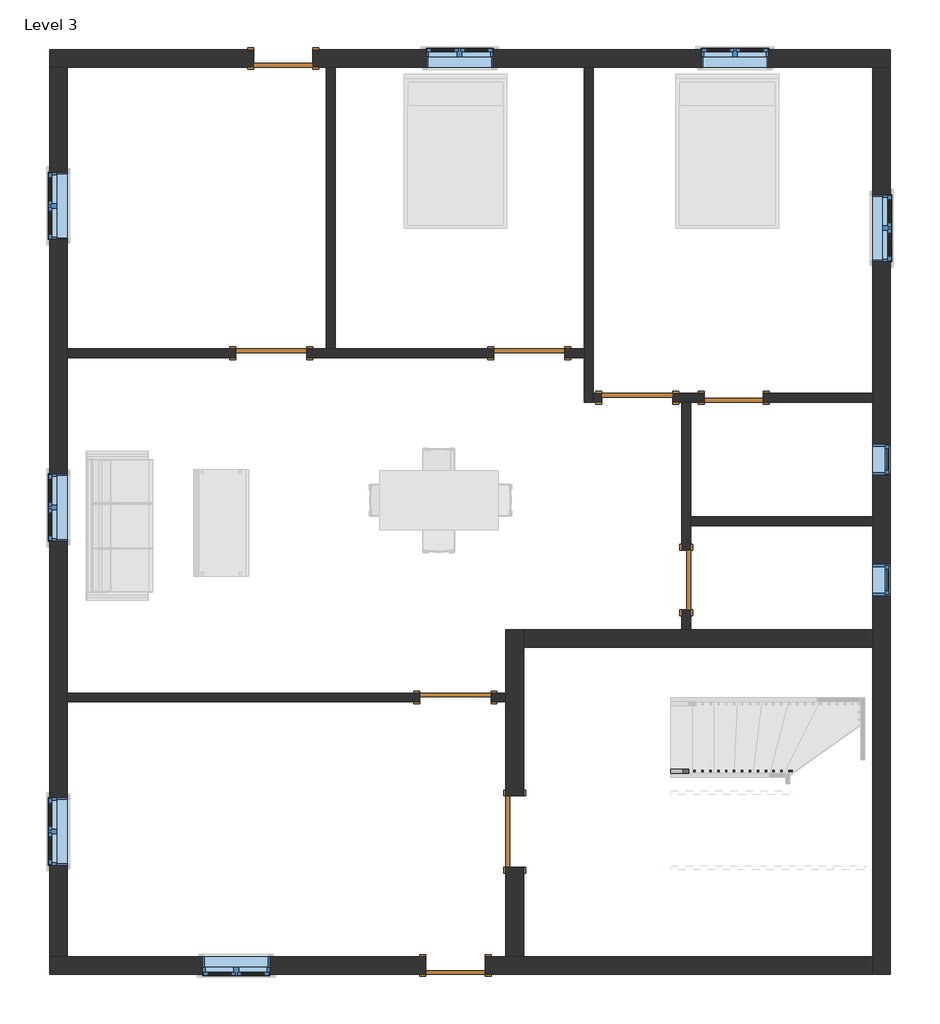
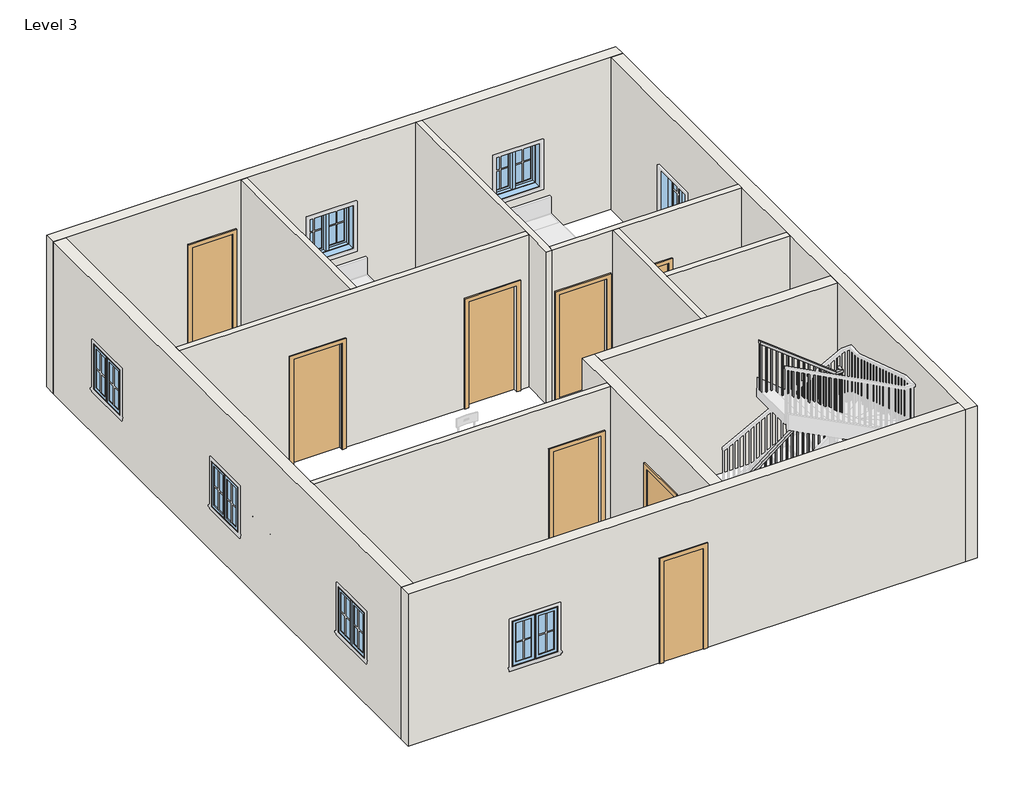
# One storey, part 1 of 2: 13 walls, 9 doors, 9 windows, 1 railing.
"""IFC4 building model written with IfcOpenShell, lengths in millimetres."""

from ifc_helpers import new_model, si_unit, frame, origin, place, context, project, spatial, polyline, outline, extrude, faceted_brep, transform, mapped, element, save
from components import door_85036156, door_d8f5dbb5, door_a1484949, door_e5f9f3c4, door_305aa2a5, door_0ca8825f, window_aa618e30, window_339605e1

model = new_model("IFC4")

# Units and contexts
model_context = context("Model", 3, world=origin())
ifc_project = project(units=[si_unit("LENGTHUNIT", "METRE", prefix="MILLI")], contexts=[model_context])

# Site, building, storey
site = spatial("IfcSite", under=ifc_project)
building = spatial("IfcBuilding", under=site)
storey = spatial("IfcBuildingStorey", under=building, Name="Level 3", Elevation=3200.4)

# Doors
placement = place(None, origin())
door_shape = door_85036156(model_context)
element("IfcDoor", 1, ObjectType="Single-Flush : 30\" x 80\"", at=placement, inside=storey, context=model_context, shape_type="MappedRepresentation", body=[
    mapped(door_shape, transform((-3639.3817864, 7024.9034997, 3200.4), x_axis=(1.0, 0.0, 0.0), y_axis=(0.0, 1.0, 0.0), z_axis=(0.0, 0.0, 1.0))),
])
door_2_shape = door_d8f5dbb5(model_context)
element("IfcDoor", 2, ObjectType="Single-Flush : 30\" x 80\"", at=placement, inside=storey, context=model_context, shape_type="MappedRepresentation", body=[
    mapped(door_2_shape, transform((2149.2782136, 2662.4534997, 3200.4), x_axis=(-1.0, 0.0, 0.0), y_axis=(0.0, -1.0, 0.0), z_axis=(0.0, 0.0, 1.0))),
])
element("IfcDoor", 3, ObjectType="Single-Flush : 30\" x 80\"", at=placement, inside=storey, context=model_context, shape_type="MappedRepresentation", body=[
    mapped(door_2_shape, transform((1539.6782136, 322.4784997, 3200.4), x_axis=(0.0, -1.0, 0.0), y_axis=(1.0, 0.0, 0.0), z_axis=(0.0, 0.0, 1.0))),
])
door_3_shape = door_a1484949(model_context)
element("IfcDoor", 4, ObjectType="Single-Flush : 30\" x 80\"", at=placement, inside=storey, context=model_context, shape_type="MappedRepresentation", body=[
    mapped(door_3_shape, transform((-1425.7717864, -4633.6965003, 3200.4), x_axis=(-1.0, 0.0, 0.0), y_axis=(0.0, -1.0, 0.0), z_axis=(0.0, 0.0, 1.0))),
])
door_4_shape = door_e5f9f3c4(model_context)
element("IfcDoor", 5, ObjectType="Single-Flush : 36\" x 84\"", at=placement, inside=storey, context=model_context, shape_type="MappedRepresentation", body=[
    mapped(door_4_shape, transform((-477.0817864, 3233.9534997, 3200.4), x_axis=(1.0, 0.0, 0.0), y_axis=(0.0, 1.0, 0.0), z_axis=(0.0, 0.0, 1.0))),
])
element("IfcDoor", 6, ObjectType="Single-Flush : 36\" x 84\"", at=placement, inside=storey, context=model_context, shape_type="MappedRepresentation", body=[
    mapped(door_4_shape, transform((-3791.7817864, 3233.9534997, 3200.4), x_axis=(1.0, 0.0, 0.0), y_axis=(0.0, 1.0, 0.0), z_axis=(0.0, 0.0, 1.0))),
])
element("IfcDoor", 7, ObjectType="Single-Flush : 36\" x 84\"", at=placement, inside=storey, context=model_context, shape_type="MappedRepresentation", body=[
    mapped(door_4_shape, transform((-1425.7717864, -1188.1865003, 3200.4), x_axis=(1.0, 0.0, 0.0), y_axis=(0.0, 1.0, 0.0), z_axis=(0.0, 0.0, 1.0))),
])
door_5_shape = door_305aa2a5(model_context)
element("IfcDoor", 8, ObjectType="Single-Flush : 36\" x 84\"", at=placement, inside=storey, context=model_context, shape_type="MappedRepresentation", body=[
    mapped(door_5_shape, transform((912.2982136, 2662.4534997, 3200.4), x_axis=(-1.0, 0.0, 0.0), y_axis=(0.0, -1.0, 0.0), z_axis=(0.0, 0.0, 1.0))),
])
door_6_shape = door_0ca8825f(model_context)
element("IfcDoor", 9, ObjectType="Single-Flush : 36\" x 84\"", at=placement, inside=storey, context=model_context, shape_type="MappedRepresentation", body=[
    mapped(door_6_shape, transform((-663.7717864, -2910.9415003, 3200.4), x_axis=(0.0, 1.0, 0.0), y_axis=(-1.0, 0.0, 0.0), z_axis=(0.0, 0.0, 1.0))),
])

# Railing
element("IfcRailing", 10, ObjectType="Handrail - Rectangular", at=placement, inside=storey, context=model_context, shape_type="SolidModel", body=[
    faceted_brep([(1342.8282136, -2108.9365003, 4284.1333333), (1342.8282136, -2108.9365003, 4219.8000346), (1342.8282136, -2159.7365003, 4219.8000346), (1342.8282136, -2159.7365003, 4284.1333333), (2794.3599055, -2108.9365003, 5412.0191036), (2845.1599055, -2108.9365003, 5387.1590024), (2845.1599055, -2159.7365003, 5387.1590024), (2794.3599055, -2159.7365003, 5412.0191036), (2794.3599055, -2108.9365003, 5615.0281882), (2845.1599055, -2108.9365003, 5564.2281882), (2845.1599055, -2159.7365003, 5564.2281882), (2794.3599055, -2159.7365003, 5615.0281882), (2921.3599055, -2108.9365003, 5615.0281882), (2921.3599055, -2108.9365003, 5564.2281882), (2870.5599055, -2159.7365003, 5564.2281882), (2870.5599055, -2159.7365003, 5615.0281882), (2921.3599055, -2235.9365003, 5615.0281882), (2921.3599055, -2265.0578342, 5564.2281882), (2870.5599055, -2265.0578342, 5564.2281882), (2870.5599055, -2235.9365003, 5615.0281882), (2921.3599055, -2362.9365003, 5831.9051451), (2921.3599055, -2413.7365003, 5818.1256424), (2870.5599055, -2413.7365003, 5818.1256424), (2870.5599055, -2362.9365003, 5831.9051451), (2921.3599055, -2362.9365003, 6034.9142297), (2921.3599055, -2413.7365003, 5984.1142297), (2870.5599055, -2413.7365003, 5984.1142297), (2870.5599055, -2362.9365003, 6034.9142297), (2921.3599055, -2489.9365003, 6034.9142297), (2921.3599055, -2489.9365003, 5984.1142297), (2870.5599055, -2439.1365003, 5984.1142297), (2870.5599055, -2439.1365003, 6034.9142297), (2794.3599055, -2489.9365003, 6034.9142297), (2776.9432376, -2489.9365003, 5984.1142297), (2776.9432376, -2439.1365003, 5984.1142297), (2794.3599055, -2439.1365003, 6034.9142297), (1342.8282136, -2489.9365003, 7162.8), (1342.8282136, -2439.1365003, 7162.8), (1342.8282136, -2439.1365003, 7098.4667013), (1342.8282136, -2489.9365003, 7098.4667013)], [[[0, 1, 2, 3]], [[1, 0, 4, 5]], [[2, 1, 5, 6]], [[3, 2, 6, 7]], [[0, 3, 7, 4]], [[5, 4, 8, 9]], [[6, 5, 9, 10]], [[7, 6, 10, 11]], [[4, 7, 11, 8]], [[9, 8, 12, 13]], [[10, 9, 13, 14]], [[11, 10, 14, 15]], [[8, 11, 15, 12]], [[13, 12, 16, 17]], [[14, 13, 17, 18]], [[15, 14, 18, 19]], [[12, 15, 19, 16]], [[17, 16, 20, 21]], [[18, 17, 21, 22]], [[19, 18, 22, 23]], [[16, 19, 23, 20]], [[21, 20, 24, 25]], [[22, 21, 25, 26]], [[23, 22, 26, 27]], [[20, 23, 27, 24]], [[25, 24, 28, 29]], [[26, 25, 29, 30]], [[27, 26, 30, 31]], [[24, 27, 31, 28]], [[29, 28, 32, 33]], [[30, 29, 33, 34]], [[31, 30, 34, 35]], [[28, 31, 35, 32]], [[36, 37, 38, 39]], [[33, 32, 36, 39]], [[34, 33, 39, 38]], [[35, 34, 38, 37]], [[32, 35, 37, 36]]]),
    extrude(outline(polyline([(7068.4292361, 1381.4849055), (7083.2316852, 1362.4349055), (6079.0666667, 1362.4349055), (6079.0666667, 1381.4849055), (7068.4292361, 1381.4849055)])), frame((0.0, -2474.0615003, 0.0), z_axis=(0.0, 1.0, 0.0), x_axis=(0.0, 0.0, 1.0)), (0.0, 0.0, 1.0), 19.05),
    extrude(outline(polyline([(6989.4828411, 1483.0849055), (7004.2852902, 1464.0349055), (6079.0666667, 1464.0349055), (6079.0666667, 1483.0849055), (6989.4828411, 1483.0849055)])), frame((0.0, -2474.0615003, 0.0), z_axis=(0.0, 1.0, 0.0), x_axis=(0.0, 0.0, 1.0)), (0.0, 0.0, 1.0), 19.05),
    extrude(outline(polyline([(6910.5364462, 1584.6849055), (6925.3388952, 1565.6349055), (6079.0666667, 1565.6349055), (6079.0666667, 1584.6849055), (6910.5364462, 1584.6849055)])), frame((0.0, -2474.0615003, 0.0), z_axis=(0.0, 1.0, 0.0), x_axis=(0.0, 0.0, 1.0)), (0.0, 0.0, 1.0), 19.05),
    extrude(outline(polyline([(6831.5900512, 1686.2849055), (6846.3925003, 1667.2349055), (5909.7333333, 1667.2349055), (5909.7333333, 1686.2849055), (6831.5900512, 1686.2849055)])), frame((0.0, -2474.0615003, 0.0), z_axis=(0.0, 1.0, 0.0), x_axis=(0.0, 0.0, 1.0)), (0.0, 0.0, 1.0), 19.05),
    extrude(outline(polyline([(6752.6436562, 1787.8849055), (6767.4461053, 1768.8349055), (5909.7333333, 1768.8349055), (5909.7333333, 1787.8849055), (6752.6436562, 1787.8849055)])), frame((0.0, -2474.0615003, 0.0), z_axis=(0.0, 1.0, 0.0), x_axis=(0.0, 0.0, 1.0)), (0.0, 0.0, 1.0), 19.05),
    extrude(outline(polyline([(6673.6972613, 1889.4849055), (6688.4997103, 1870.4349055), (5909.7333333, 1870.4349055), (5909.7333333, 1889.4849055), (6673.6972613, 1889.4849055)])), frame((0.0, -2474.0615003, 0.0), z_axis=(0.0, 1.0, 0.0), x_axis=(0.0, 0.0, 1.0)), (0.0, 0.0, 1.0), 19.05),
    extrude(outline(polyline([(6594.7508663, 1991.0849055), (6609.5533154, 1972.0349055), (5740.4, 1972.0349055), (5740.4, 1991.0849055), (6594.7508663, 1991.0849055)])), frame((0.0, -2474.0615003, 0.0), z_axis=(0.0, 1.0, 0.0), x_axis=(0.0, 0.0, 1.0)), (0.0, 0.0, 1.0), 19.05),
    extrude(outline(polyline([(6515.8044713, 2092.6849055), (6530.6069204, 2073.6349055), (5740.4, 2073.6349055), (5740.4, 2092.6849055), (6515.8044713, 2092.6849055)])), frame((0.0, -2474.0615003, 0.0), z_axis=(0.0, 1.0, 0.0), x_axis=(0.0, 0.0, 1.0)), (0.0, 0.0, 1.0), 19.05),
    extrude(outline(polyline([(6436.8580764, 2194.2849055), (6451.6605254, 2175.2349055), (5571.0666667, 2175.2349055), (5571.0666667, 2194.2849055), (6436.8580764, 2194.2849055)])), frame((0.0, -2474.0615003, 0.0), z_axis=(0.0, 1.0, 0.0), x_axis=(0.0, 0.0, 1.0)), (0.0, 0.0, 1.0), 19.05),
    extrude(outline(polyline([(6357.9116814, 2295.8849055), (6372.7141304, 2276.8349055), (5571.0666667, 2276.8349055), (5571.0666667, 2295.8849055), (6357.9116814, 2295.8849055)])), frame((0.0, -2474.0615003, 0.0), z_axis=(0.0, 1.0, 0.0), x_axis=(0.0, 0.0, 1.0)), (0.0, 0.0, 1.0), 19.05),
    extrude(outline(polyline([(6278.9652864, 2397.4849055), (6293.7677355, 2378.4349055), (5571.0666667, 2378.4349055), (5571.0666667, 2397.4849055), (6278.9652864, 2397.4849055)])), frame((0.0, -2474.0615003, 0.0), z_axis=(0.0, 1.0, 0.0), x_axis=(0.0, 0.0, 1.0)), (0.0, 0.0, 1.0), 19.05),
    extrude(outline(polyline([(6200.0188914, 2499.0849055), (6214.8213405, 2480.0349055), (5401.7333333, 2480.0349055), (5401.7333333, 2499.0849055), (6200.0188914, 2499.0849055)])), frame((0.0, -2474.0615003, 0.0), z_axis=(0.0, 1.0, 0.0), x_axis=(0.0, 0.0, 1.0)), (0.0, 0.0, 1.0), 19.05),
    extrude(outline(polyline([(6121.0724965, 2600.6849055), (6135.8749455, 2581.6349055), (5401.7333333, 2581.6349055), (5401.7333333, 2600.6849055), (6121.0724965, 2600.6849055)])), frame((0.0, -2474.0615003, 0.0), z_axis=(0.0, 1.0, 0.0), x_axis=(0.0, 0.0, 1.0)), (0.0, 0.0, 1.0), 19.05),
    extrude(outline(polyline([(6042.1261015, 2702.2849055), (6056.9285506, 2683.2349055), (5232.4, 2683.2349055), (5232.4, 2702.2849055), (6042.1261015, 2702.2849055)])), frame((0.0, -2474.0615003, 0.0), z_axis=(0.0, 1.0, 0.0), x_axis=(0.0, 0.0, 1.0)), (0.0, 0.0, 1.0), 19.05),
    extrude(outline(polyline([(5963.1797065, 2803.8849055), (5977.9821556, 2784.8349055), (5232.4, 2784.8349055), (5232.4, 2803.8849055), (5963.1797065, 2803.8849055)])), frame((0.0, -2474.0615003, 0.0), z_axis=(0.0, 1.0, 0.0), x_axis=(0.0, 0.0, 1.0)), (0.0, 0.0, 1.0), 19.05),
    extrude(outline(polyline([(2886.4349055, -2429.6115003), (2905.4849055, -2429.6115003), (2905.4849055, -2448.6615003), (2886.4349055, -2448.6615003), (2886.4349055, -2429.6115003)])), frame((0.0, 0.0, 4893.7333333), z_axis=(0.0, 0.0, 1.0), x_axis=(1.0, 0.0, 0.0)), (0.0, 0.0, 1.0), 1090.3808964),
    extrude(outline(polyline([(-2347.0615003, 5704.26524), (-2328.0115003, 5671.7336964), (-2328.0115003, 4724.4), (-2347.0615003, 4724.4), (-2347.0615003, 5704.26524)])), frame((2886.4349055, 0.0, 0.0), z_axis=(1.0, 0.0, 0.0), x_axis=(0.0, 1.0, 0.0)), (0.0, 0.0, 1.0), 19.05),
    extrude(outline(polyline([(-2245.4615003, 5530.7636744), (-2226.4115003, 5498.2321309), (-2226.4115003, 4555.0666667), (-2245.4615003, 4555.0666667), (-2245.4615003, 5530.7636744)])), frame((2886.4349055, 0.0, 0.0), z_axis=(1.0, 0.0, 0.0), x_axis=(0.0, 1.0, 0.0)), (0.0, 0.0, 1.0), 19.05),
    extrude(outline(polyline([(2857.3032136, -2143.8615003), (2857.3032136, -2124.8115003), (2876.3532136, -2124.8115003), (2876.3532136, -2143.8615003), (2857.3032136, -2143.8615003)])), frame((0.0, 0.0, 4385.7333333), z_axis=(0.0, 0.0, 1.0), x_axis=(1.0, 0.0, 0.0)), (0.0, 0.0, 1.0), 1178.4948549),
    extrude(outline(polyline([(5332.4507888, 2774.7532136), (5317.6483397, 2755.7032136), (4216.4, 2755.7032136), (4216.4, 2774.7532136), (5332.4507888, 2774.7532136)])), frame((0.0, -2143.8615003, 0.0), z_axis=(0.0, 1.0, 0.0), x_axis=(0.0, 0.0, 1.0)), (0.0, 0.0, 1.0), 19.05),
    extrude(outline(polyline([(5253.5043938, 2673.1532136), (5238.7019447, 2654.1032136), (4216.4, 2654.1032136), (4216.4, 2673.1532136), (5253.5043938, 2673.1532136)])), frame((0.0, -2143.8615003, 0.0), z_axis=(0.0, 1.0, 0.0), x_axis=(0.0, 0.0, 1.0)), (0.0, 0.0, 1.0), 19.05),
    extrude(outline(polyline([(5174.5579988, 2571.5532136), (5159.7555498, 2552.5032136), (4047.0666667, 2552.5032136), (4047.0666667, 2571.5532136), (5174.5579988, 2571.5532136)])), frame((0.0, -2143.8615003, 0.0), z_axis=(0.0, 1.0, 0.0), x_axis=(0.0, 0.0, 1.0)), (0.0, 0.0, 1.0), 19.05),
    extrude(outline(polyline([(5095.6116039, 2469.9532136), (5080.8091548, 2450.9032136), (4047.0666667, 2450.9032136), (4047.0666667, 2469.9532136), (5095.6116039, 2469.9532136)])), frame((0.0, -2143.8615003, 0.0), z_axis=(0.0, 1.0, 0.0), x_axis=(0.0, 0.0, 1.0)), (0.0, 0.0, 1.0), 19.05),
    extrude(outline(polyline([(5016.6652089, 2368.3532136), (5001.8627598, 2349.3032136), (3877.7333333, 2349.3032136), (3877.7333333, 2368.3532136), (5016.6652089, 2368.3532136)])), frame((0.0, -2143.8615003, 0.0), z_axis=(0.0, 1.0, 0.0), x_axis=(0.0, 0.0, 1.0)), (0.0, 0.0, 1.0), 19.05),
    extrude(outline(polyline([(4937.7188139, 2266.7532136), (4922.9163649, 2247.7032136), (3877.7333333, 2247.7032136), (3877.7333333, 2266.7532136), (4937.7188139, 2266.7532136)])), frame((0.0, -2143.8615003, 0.0), z_axis=(0.0, 1.0, 0.0), x_axis=(0.0, 0.0, 1.0)), (0.0, 0.0, 1.0), 19.05),
    extrude(outline(polyline([(4858.7724189, 2165.1532136), (4843.9699699, 2146.1032136), (3708.4, 2146.1032136), (3708.4, 2165.1532136), (4858.7724189, 2165.1532136)])), frame((0.0, -2143.8615003, 0.0), z_axis=(0.0, 1.0, 0.0), x_axis=(0.0, 0.0, 1.0)), (0.0, 0.0, 1.0), 19.05),
    extrude(outline(polyline([(4779.826024, 2063.5532136), (4765.0235749, 2044.5032136), (3708.4, 2044.5032136), (3708.4, 2063.5532136), (4779.826024, 2063.5532136)])), frame((0.0, -2143.8615003, 0.0), z_axis=(0.0, 1.0, 0.0), x_axis=(0.0, 0.0, 1.0)), (0.0, 0.0, 1.0), 19.05),
    extrude(outline(polyline([(4700.879629, 1961.9532136), (4686.0771799, 1942.9032136), (3708.4, 1942.9032136), (3708.4, 1961.9532136), (4700.879629, 1961.9532136)])), frame((0.0, -2143.8615003, 0.0), z_axis=(0.0, 1.0, 0.0), x_axis=(0.0, 0.0, 1.0)), (0.0, 0.0, 1.0), 19.05),
    extrude(outline(polyline([(4621.933234, 1860.3532136), (4607.130785, 1841.3032136), (3539.0666667, 1841.3032136), (3539.0666667, 1860.3532136), (4621.933234, 1860.3532136)])), frame((0.0, -2143.8615003, 0.0), z_axis=(0.0, 1.0, 0.0), x_axis=(0.0, 0.0, 1.0)), (0.0, 0.0, 1.0), 19.05),
    extrude(outline(polyline([(4542.9868391, 1758.7532136), (4528.18439, 1739.7032136), (3539.0666667, 1739.7032136), (3539.0666667, 1758.7532136), (4542.9868391, 1758.7532136)])), frame((0.0, -2143.8615003, 0.0), z_axis=(0.0, 1.0, 0.0), x_axis=(0.0, 0.0, 1.0)), (0.0, 0.0, 1.0), 19.05),
    extrude(outline(polyline([(4464.0404441, 1657.1532136), (4449.237995, 1638.1032136), (3539.0666667, 1638.1032136), (3539.0666667, 1657.1532136), (4464.0404441, 1657.1532136)])), frame((0.0, -2143.8615003, 0.0), z_axis=(0.0, 1.0, 0.0), x_axis=(0.0, 0.0, 1.0)), (0.0, 0.0, 1.0), 19.05),
    extrude(outline(polyline([(4385.0940491, 1555.5532136), (4370.2916001, 1536.5032136), (3369.7333333, 1536.5032136), (3369.7333333, 1555.5532136), (4385.0940491, 1555.5532136)])), frame((0.0, -2143.8615003, 0.0), z_axis=(0.0, 1.0, 0.0), x_axis=(0.0, 0.0, 1.0)), (0.0, 0.0, 1.0), 19.05),
    extrude(outline(polyline([(4306.1476541, 1453.9532136), (4291.3452051, 1434.9032136), (3369.7333333, 1434.9032136), (3369.7333333, 1453.9532136), (4306.1476541, 1453.9532136)])), frame((0.0, -2143.8615003, 0.0), z_axis=(0.0, 1.0, 0.0), x_axis=(0.0, 0.0, 1.0)), (0.0, 0.0, 1.0), 19.05),
    extrude(outline(polyline([(2886.4349055, -2455.0115003), (2905.4849055, -2455.0115003), (2905.4849055, -2474.0615003), (2886.4349055, -2474.0615003), (2886.4349055, -2455.0115003)])), frame((0.0, 0.0, 5063.0666667), z_axis=(0.0, 0.0, 1.0), x_axis=(1.0, 0.0, 0.0)), (0.0, 0.0, 1.0), 921.0475631),
    extrude(outline(polyline([(2886.4349055, -2143.8615003), (2886.4349055, -2124.8115003), (2905.4849055, -2124.8115003), (2905.4849055, -2143.8615003), (2886.4349055, -2143.8615003)])), frame((0.0, 0.0, 4385.7333333), z_axis=(0.0, 0.0, 1.0), x_axis=(1.0, 0.0, 0.0)), (0.0, 0.0, 1.0), 1178.4948549),
    extrude(outline(polyline([(7083.6642523, 1361.8782136), (7098.4667013, 1342.8282136), (6079.0666667, 1342.8282136), (6079.0666667, 1361.8782136), (7083.6642523, 1361.8782136)])), frame((0.0, -2474.0615003, 0.0), z_axis=(0.0, 1.0, 0.0), x_axis=(0.0, 0.0, 1.0)), (0.0, 0.0, 1.0), 19.05),
    extrude(outline(polyline([(4234.6024837, 1361.8782136), (4219.8000346, 1342.8282136), (3369.7333333, 1342.8282136), (3369.7333333, 1361.8782136), (4234.6024837, 1361.8782136)])), frame((0.0, -2143.8615003, 0.0), z_axis=(0.0, 1.0, 0.0), x_axis=(0.0, 0.0, 1.0)), (0.0, 0.0, 1.0), 19.05),
])

# Walls
element("IfcWall", 11, ObjectType="WALL4.5\"", at=placement, inside=storey, context=model_context, shape_type="Brep", body=[
    faceted_brep([(-3334.5817864, 3176.8034997, 5334.0), (-3334.5817864, 3176.8034997, 3200.4), (-934.2817864, 3176.8034997, 3200.4), (-934.2817864, 3176.8034997, 5334.0), (-19.8817864, 3176.8034997, 5334.0), (-19.8817864, 3176.8034997, 3200.4), (227.7682136, 3176.8034997, 3200.4), (227.7682136, 3176.8034997, 6248.4), (-6414.3317864, 3176.8034997, 6248.4), (-6414.3317864, 3176.8034997, 3200.4), (-4248.9817864, 3176.8034997, 3200.4), (-4248.9817864, 3176.8034997, 5334.0), (-934.2817864, 3291.1034997, 3200.4), (-2972.6317864, 3291.1034997, 3200.4), (-3086.9317864, 3291.1034997, 3200.4), (-3334.5817864, 3291.1034997, 3200.4), (-3334.5817864, 3291.1034997, 5334.0), (-4248.9817864, 3291.1034997, 5334.0), (-4248.9817864, 3291.1034997, 3200.4), (-6414.3317864, 3291.1034997, 3200.4), (-6414.3317864, 3291.1034997, 6248.4), (-3086.9317864, 3291.1034997, 6248.4), (-2972.6317864, 3291.1034997, 6248.4), (227.7682136, 3291.1034997, 6248.4), (227.7682136, 3291.1034997, 3200.4), (-19.8817864, 3291.1034997, 3200.4), (-19.8817864, 3291.1034997, 5334.0), (-934.2817864, 3291.1034997, 5334.0)], [[[0, 1, 2, 3, 4, 5, 6, 7, 8, 9, 10, 11]], [[12, 13, 14, 15, 16, 17, 18, 19, 20, 21, 22, 23, 24, 25, 26, 27]], [[6, 5, 25, 24]], [[10, 9, 19, 18]], [[2, 1, 15, 14, 13, 12]], [[9, 8, 20, 19]], [[7, 6, 24, 23]], [[26, 25, 5, 4]], [[27, 26, 4, 3]], [[12, 27, 3, 2]], [[16, 15, 1, 0]], [[17, 16, 0, 11]], [[18, 17, 11, 10]], [[8, 7, 23, 22, 21, 20]]]),
])
element("IfcWall", 12, ObjectType="WALL4.5\"", at=placement, inside=storey, context=model_context, shape_type="Brep", body=[
    faceted_brep([(227.7682136, 6910.6034997, 3200.4), (227.7682136, 3291.1034997, 3200.4), (227.7682136, 3176.8034997, 3200.4), (227.7682136, 2605.3034997, 3200.4), (227.7682136, 2605.3034997, 6248.4), (227.7682136, 3176.8034997, 6248.4), (227.7682136, 3291.1034997, 6248.4), (227.7682136, 6910.6034997, 6248.4), (342.0682136, 6910.6034997, 3200.4), (342.0682136, 6910.6034997, 6248.4), (342.0682136, 2719.6034997, 6248.4), (342.0682136, 2605.3034997, 6248.4), (342.0682136, 2605.3034997, 3200.4), (342.0682136, 2719.6034997, 3200.4)], [[[0, 1, 2, 3, 4, 5, 6, 7]], [[8, 9, 10, 11, 12, 13]], [[3, 2, 1, 0, 8, 13, 12]], [[0, 7, 9, 8]], [[4, 3, 12, 11]], [[7, 6, 5, 4, 11, 10, 9]]]),
])
element("IfcWall", 13, ObjectType="WALL4.5\"", at=placement, inside=storey, context=model_context, shape_type="Brep", body=[
    faceted_brep([(1369.4982136, 2605.3034997, 3200.4), (1482.5282136, 2605.3034997, 3200.4), (1596.8282136, 2605.3034997, 3200.4), (1768.2782136, 2605.3034997, 3200.4), (1768.2782136, 2605.3034997, 5232.4), (2530.2782136, 2605.3034997, 5232.4), (2530.2782136, 2605.3034997, 3200.4), (3933.6282136, 2605.3034997, 3200.4), (3933.6282136, 2605.3034997, 6248.4), (1596.8282136, 2605.3034997, 6248.4), (1482.5282136, 2605.3034997, 6248.4), (342.0682136, 2605.3034997, 6248.4), (342.0682136, 2605.3034997, 3200.4), (455.0982136, 2605.3034997, 3200.4), (455.0982136, 2605.3034997, 5334.0), (1369.4982136, 2605.3034997, 5334.0), (1768.2782136, 2719.6034997, 5232.4), (1768.2782136, 2719.6034997, 3200.4), (1369.4982136, 2719.6034997, 3200.4), (1369.4982136, 2719.6034997, 5334.0), (455.0982136, 2719.6034997, 5334.0), (455.0982136, 2719.6034997, 3200.4), (342.0682136, 2719.6034997, 3200.4), (342.0682136, 2719.6034997, 6248.4), (3933.6282136, 2719.6034997, 6248.4), (3933.6282136, 2719.6034997, 3200.4), (2530.2782136, 2719.6034997, 3200.4), (2530.2782136, 2719.6034997, 5232.4)], [[[0, 1, 2, 3, 4, 5, 6, 7, 8, 9, 10, 11, 12, 13, 14, 15]], [[16, 17, 18, 19, 20, 21, 22, 23, 24, 25, 26, 27]], [[22, 21, 13, 12]], [[26, 25, 7, 6]], [[18, 17, 3, 2, 1, 0]], [[12, 11, 23, 22]], [[8, 7, 25, 24]], [[14, 13, 21, 20]], [[15, 14, 20, 19]], [[0, 15, 19, 18]], [[4, 3, 17, 16]], [[5, 4, 16, 27]], [[6, 5, 27, 26]], [[11, 10, 9, 8, 24, 23]]]),
])
element("IfcWall", 14, ObjectType="WALL4.5\"", at=placement, inside=storey, context=model_context, shape_type="SweptSolid", body=[
    extrude(outline(polyline([(-3086.9317864, 3291.1034997), (-3086.9317864, 6910.6034997), (-2972.6317864, 6910.6034997), (-2972.6317864, 3291.1034997), (-3086.9317864, 3291.1034997)])), frame((0.0, 0.0, 3200.4), z_axis=(0.0, 0.0, 1.0), x_axis=(1.0, 0.0, 0.0)), (0.0, 0.0, 1.0), 3048.0),
])
element("IfcWall", 15, ObjectType="WALL4.5\"", at=placement, inside=storey, context=model_context, shape_type="Brep", body=[
    faceted_brep([(1482.5282136, -58.5215003, 5232.4), (1482.5282136, -58.5215003, 3200.4), (1482.5282136, -315.6965003, 3200.4), (1482.5282136, -315.6965003, 6248.4), (1482.5282136, 2605.3034997, 6248.4), (1482.5282136, 2605.3034997, 3200.4), (1482.5282136, 703.4784997, 3200.4), (1482.5282136, 703.4784997, 5232.4), (1596.8282136, -315.6965003, 3200.4), (1596.8282136, -58.5215003, 3200.4), (1596.8282136, -58.5215003, 5232.4), (1596.8282136, 703.4784997, 5232.4), (1596.8282136, 703.4784997, 3200.4), (1596.8282136, 1017.8034997, 3200.4), (1596.8282136, 1132.1034997, 3200.4), (1596.8282136, 2605.3034997, 3200.4), (1596.8282136, 2605.3034997, 6248.4), (1596.8282136, 1132.1034997, 6248.4), (1596.8282136, 1017.8034997, 6248.4), (1596.8282136, -315.6965003, 6248.4)], [[[0, 1, 2, 3, 4, 5, 6, 7]], [[8, 9, 10, 11, 12, 13, 14, 15, 16, 17, 18, 19]], [[6, 5, 15, 14, 13, 12]], [[2, 1, 9, 8]], [[5, 4, 16, 15]], [[3, 2, 8, 19]], [[10, 9, 1, 0]], [[11, 10, 0, 7]], [[12, 11, 7, 6]], [[4, 3, 19, 18, 17, 16]]]),
])
element("IfcWall", 16, ObjectType="WALL4.5\"", at=placement, inside=storey, context=model_context, shape_type="SweptSolid", body=[
    extrude(outline(polyline([(3933.6282136, 1017.8034997), (1596.8282136, 1017.8034997), (1596.8282136, 1132.1034997), (3933.6282136, 1132.1034997), (3933.6282136, 1017.8034997)])), frame((0.0, 0.0, 3200.4), z_axis=(0.0, 0.0, 1.0), x_axis=(1.0, 0.0, 0.0)), (0.0, 0.0, 1.0), 3048.0),
])
element("IfcWall", 17, ObjectType="WALL4.5\"", at=placement, inside=storey, context=model_context, shape_type="SweptSolid", body=[
    extrude(outline(polyline([(5334.0, -968.5717864), (3200.4, -968.5717864), (3200.4, -778.0717864), (6248.4, -778.0717864), (6248.4, -6414.3317864), (3200.4, -6414.3317864), (3200.4, -1882.9717864), (5334.0, -1882.9717864), (5334.0, -968.5717864)])), frame((0.0, -1245.3365003, 0.0), z_axis=(0.0, 1.0, 0.0), x_axis=(0.0, 0.0, 1.0)), (0.0, 0.0, 1.0), 114.3),
])
element("IfcWall", 18, ObjectType="WALL9\"", at=placement, inside=storey, context=model_context, shape_type="Brep", body=[
    faceted_brep([(-3258.3817864, 6910.6034997, 5232.4), (-3258.3817864, 6910.6034997, 3200.4), (-3086.9317864, 6910.6034997, 3200.4), (-2972.6317864, 6910.6034997, 3200.4), (227.7682136, 6910.6034997, 3200.4), (342.0682136, 6910.6034997, 3200.4), (3933.6282136, 6910.6034997, 3200.4), (4162.2282136, 6910.6034997, 3200.4), (4162.2282136, 6910.6034997, 6248.4), (3933.6282136, 6910.6034997, 6248.4), (342.0682136, 6910.6034997, 6248.4), (227.7682136, 6910.6034997, 6248.4), (-2972.6317864, 6910.6034997, 6248.4), (-3086.9317864, 6910.6034997, 6248.4), (-6414.3317864, 6910.6034997, 6248.4), (-6642.9317864, 6910.6034997, 6248.4), (-6642.9317864, 6910.6034997, 3200.4), (-6414.3317864, 6910.6034997, 3200.4), (-4020.3817864, 6910.6034997, 3200.4), (-4020.3817864, 6910.6034997, 5232.4), (-940.6317864, 6910.6034997, 5029.2), (-940.6317864, 6910.6034997, 4114.8), (-1804.2317864, 6910.6034997, 4114.8), (-1804.2317864, 6910.6034997, 5029.2), (2598.2232136, 6910.6034997, 5029.2), (2598.2232136, 6910.6034997, 4114.8), (1734.6232136, 6910.6034997, 4114.8), (1734.6232136, 6910.6034997, 5029.2), (4162.2282136, 7139.2034997, 3200.4), (-3258.3817864, 7139.2034997, 3200.4), (-3258.3817864, 7139.2034997, 5232.4), (-4020.3817864, 7139.2034997, 5232.4), (-4020.3817864, 7139.2034997, 3200.4), (-6642.9317864, 7139.2034997, 3200.4), (-6642.9317864, 7139.2034997, 6248.4), (4162.2282136, 7139.2034997, 6248.4), (-940.6317864, 7139.2034997, 5029.2), (-1804.2317864, 7139.2034997, 5029.2), (-1804.2317864, 7139.2034997, 4114.8), (-940.6317864, 7139.2034997, 4114.8), (2598.2232136, 7139.2034997, 5029.2), (1734.6232136, 7139.2034997, 5029.2), (1734.6232136, 7139.2034997, 4114.8), (2598.2232136, 7139.2034997, 4114.8)], [[[0, 1, 2, 3, 4, 5, 6, 7, 8, 9, 10, 11, 12, 13, 14, 15, 16, 17, 18, 19], [20, 21, 22, 23], [24, 25, 26, 27]], [[28, 29, 30, 31, 32, 33, 34, 35], [36, 37, 38, 39], [40, 41, 42, 43]], [[18, 17, 16, 33, 32]], [[7, 6, 5, 4, 3, 2, 1, 29, 28]], [[8, 7, 28, 35]], [[16, 15, 34, 33]], [[30, 29, 1, 0]], [[31, 30, 0, 19]], [[32, 31, 19, 18]], [[21, 20, 36, 39]], [[22, 21, 39, 38]], [[23, 22, 38, 37]], [[20, 23, 37, 36]], [[25, 24, 40, 43]], [[26, 25, 43, 42]], [[27, 26, 42, 41]], [[24, 27, 41, 40]], [[15, 14, 13, 12, 11, 10, 9, 8, 35, 34]]]),
])
element("IfcWall", 19, ObjectType="WALL9\"", at=placement, inside=storey, context=model_context, shape_type="Brep", body=[
    faceted_brep([(3933.6282136, 6910.6034997, 3200.4), (3933.6282136, 2719.6034997, 3200.4), (3933.6282136, 2605.3034997, 3200.4), (3933.6282136, 1132.1034997, 3200.4), (3933.6282136, 1017.8034997, 3200.4), (3933.6282136, -315.6965003, 3200.4), (3933.6282136, -544.2965003, 3200.4), (3933.6282136, -4519.3965003, 3200.4), (3933.6282136, -4747.9965003, 3200.4), (3933.6282136, -4747.9965003, 6248.4), (3933.6282136, -4519.3965003, 6248.4), (3933.6282136, -544.2965003, 6248.4), (3933.6282136, -315.6965003, 6248.4), (3933.6282136, 1017.8034997, 6248.4), (3933.6282136, 1132.1034997, 6248.4), (3933.6282136, 2605.3034997, 6248.4), (3933.6282136, 2719.6034997, 6248.4), (3933.6282136, 6910.6034997, 6248.4), (3933.6282136, 1665.5034997, 4724.4), (3933.6282136, 1665.5034997, 4114.8), (3933.6282136, 2071.9034997, 4114.8), (3933.6282136, 2071.9034997, 4724.4), (3933.6282136, 119.2784997, 4724.4), (3933.6282136, 119.2784997, 4114.8), (3933.6282136, 525.6784997, 4114.8), (3933.6282136, 525.6784997, 4724.4), (3933.6282136, 4411.8784997, 5029.2), (3933.6282136, 4411.8784997, 4114.8), (3933.6282136, 5275.4784997, 4114.8), (3933.6282136, 5275.4784997, 5029.2), (4162.2282136, 6910.6034997, 3200.4), (4162.2282136, 6910.6034997, 6248.4), (4162.2282136, -4747.9965003, 6248.4), (4162.2282136, -4747.9965003, 3200.4), (4162.2282136, 1665.5034997, 4724.4), (4162.2282136, 2071.9034997, 4724.4), (4162.2282136, 2071.9034997, 4114.8), (4162.2282136, 1665.5034997, 4114.8), (4162.2282136, 119.2784997, 4724.4), (4162.2282136, 525.6784997, 4724.4), (4162.2282136, 525.6784997, 4114.8), (4162.2282136, 119.2784997, 4114.8), (4162.2282136, 4411.8784997, 5029.2), (4162.2282136, 5275.4784997, 5029.2), (4162.2282136, 5275.4784997, 4114.8), (4162.2282136, 4411.8784997, 4114.8)], [[[0, 1, 2, 3, 4, 5, 6, 7, 8, 9, 10, 11, 12, 13, 14, 15, 16, 17], [18, 19, 20, 21], [22, 23, 24, 25], [26, 27, 28, 29]], [[30, 31, 32, 33], [34, 35, 36, 37], [38, 39, 40, 41], [42, 43, 44, 45]], [[8, 7, 6, 5, 4, 3, 2, 1, 0, 30, 33]], [[0, 17, 31, 30]], [[9, 8, 33, 32]], [[19, 18, 34, 37]], [[20, 19, 37, 36]], [[21, 20, 36, 35]], [[18, 21, 35, 34]], [[23, 22, 38, 41]], [[24, 23, 41, 40]], [[25, 24, 40, 39]], [[22, 25, 39, 38]], [[27, 26, 42, 45]], [[28, 27, 45, 44]], [[29, 28, 44, 43]], [[26, 29, 43, 42]], [[17, 16, 15, 14, 13, 12, 11, 10, 9, 32, 31]]]),
])
element("IfcWall", 20, ObjectType="WALL9\"", at=placement, inside=storey, context=model_context, shape_type="Brep", body=[
    faceted_brep([(-1806.7717864, -4519.3965003, 5232.4), (-1806.7717864, -4519.3965003, 3200.4), (-6414.3317864, -4519.3965003, 3200.4), (-6642.9317864, -4519.3965003, 3200.4), (-6642.9317864, -4519.3965003, 6248.4), (-6414.3317864, -4519.3965003, 6248.4), (-778.0717864, -4519.3965003, 6248.4), (-549.4717864, -4519.3965003, 6248.4), (3933.6282136, -4519.3965003, 6248.4), (3933.6282136, -4519.3965003, 3200.4), (-549.4717864, -4519.3965003, 3200.4), (-778.0717864, -4519.3965003, 3200.4), (-1044.7717864, -4519.3965003, 3200.4), (-1044.7717864, -4519.3965003, 5232.4), (-4674.4317864, -4519.3965003, 5029.2), (-4674.4317864, -4519.3965003, 4114.8), (-3810.8317864, -4519.3965003, 4114.8), (-3810.8317864, -4519.3965003, 5029.2), (-6642.9317864, -4747.9965003, 3200.4), (-1806.7717864, -4747.9965003, 3200.4), (-1806.7717864, -4747.9965003, 5232.4), (-1044.7717864, -4747.9965003, 5232.4), (-1044.7717864, -4747.9965003, 3200.4), (3933.6282136, -4747.9965003, 3200.4), (3933.6282136, -4747.9965003, 6248.4), (-6642.9317864, -4747.9965003, 6248.4), (-4674.4317864, -4747.9965003, 5029.2), (-3810.8317864, -4747.9965003, 5029.2), (-3810.8317864, -4747.9965003, 4114.8), (-4674.4317864, -4747.9965003, 4114.8)], [[[0, 1, 2, 3, 4, 5, 6, 7, 8, 9, 10, 11, 12, 13], [14, 15, 16, 17]], [[18, 19, 20, 21, 22, 23, 24, 25], [26, 27, 28, 29]], [[3, 2, 1, 19, 18]], [[12, 11, 10, 9, 23, 22]], [[9, 8, 24, 23]], [[4, 3, 18, 25]], [[15, 14, 26, 29]], [[16, 15, 29, 28]], [[17, 16, 28, 27]], [[14, 17, 27, 26]], [[8, 7, 6, 5, 4, 25, 24]], [[20, 19, 1, 0]], [[21, 20, 0, 13]], [[22, 21, 13, 12]]]),
])
element("IfcWall", 21, ObjectType="WALL9\"", at=placement, inside=storey, context=model_context, shape_type="Brep", body=[
    faceted_brep([(-6414.3317864, -4519.3965003, 3200.4), (-6414.3317864, -1245.3365003, 3200.4), (-6414.3317864, -1131.0365003, 3200.4), (-6414.3317864, 3176.8034997, 3200.4), (-6414.3317864, 3291.1034997, 3200.4), (-6414.3317864, 6910.6034997, 3200.4), (-6414.3317864, 6910.6034997, 6248.4), (-6414.3317864, 3291.1034997, 6248.4), (-6414.3317864, 3176.8034997, 6248.4), (-6414.3317864, -1131.0365003, 6248.4), (-6414.3317864, -1245.3365003, 6248.4), (-6414.3317864, -4519.3965003, 6248.4), (-6414.3317864, 5561.2284997, 5029.2), (-6414.3317864, 5561.2284997, 4114.8), (-6414.3317864, 4697.6284997, 4114.8), (-6414.3317864, 4697.6284997, 5029.2), (-6414.3317864, 1684.5534997, 5029.2), (-6414.3317864, 1684.5534997, 4114.8), (-6414.3317864, 820.9534997, 4114.8), (-6414.3317864, 820.9534997, 5029.2), (-6414.3317864, -2479.1415003, 5029.2), (-6414.3317864, -2479.1415003, 4114.8), (-6414.3317864, -3342.7415003, 4114.8), (-6414.3317864, -3342.7415003, 5029.2), (-6642.9317864, -4519.3965003, 3200.4), (-6642.9317864, -4519.3965003, 6248.4), (-6642.9317864, 6910.6034997, 6248.4), (-6642.9317864, 6910.6034997, 3200.4), (-6642.9317864, 5561.2284997, 5029.2), (-6642.9317864, 4697.6284997, 5029.2), (-6642.9317864, 4697.6284997, 4114.8), (-6642.9317864, 5561.2284997, 4114.8), (-6642.9317864, 1684.5534997, 5029.2), (-6642.9317864, 820.9534997, 5029.2), (-6642.9317864, 820.9534997, 4114.8), (-6642.9317864, 1684.5534997, 4114.8), (-6642.9317864, -2479.1415003, 5029.2), (-6642.9317864, -3342.7415003, 5029.2), (-6642.9317864, -3342.7415003, 4114.8), (-6642.9317864, -2479.1415003, 4114.8)], [[[0, 1, 2, 3, 4, 5, 6, 7, 8, 9, 10, 11], [12, 13, 14, 15], [16, 17, 18, 19], [20, 21, 22, 23]], [[24, 25, 26, 27], [28, 29, 30, 31], [32, 33, 34, 35], [36, 37, 38, 39]], [[5, 4, 3, 2, 1, 0, 24, 27]], [[0, 11, 25, 24]], [[6, 5, 27, 26]], [[13, 12, 28, 31]], [[14, 13, 31, 30]], [[15, 14, 30, 29]], [[12, 15, 29, 28]], [[17, 16, 32, 35]], [[18, 17, 35, 34]], [[19, 18, 34, 33]], [[16, 19, 33, 32]], [[21, 20, 36, 39]], [[22, 21, 39, 38]], [[23, 22, 38, 37]], [[20, 23, 37, 36]], [[11, 10, 9, 8, 7, 6, 26, 25]]]),
])
element("IfcWall", 22, ObjectType="WALL9\"", at=placement, inside=storey, context=model_context, shape_type="Brep", body=[
    faceted_brep([(-549.4717864, -2453.7415003, 5334.0), (-549.4717864, -2453.7415003, 3200.4), (-549.4717864, -544.2965003, 3200.4), (-549.4717864, -315.6965003, 3200.4), (-549.4717864, -315.6965003, 6248.4), (-549.4717864, -544.2965003, 6248.4), (-549.4717864, -4519.3965003, 6248.4), (-549.4717864, -4519.3965003, 3200.4), (-549.4717864, -3368.1415003, 3200.4), (-549.4717864, -3368.1415003, 5334.0), (-778.0717864, -315.6965003, 3200.4), (-778.0717864, -1131.0365003, 3200.4), (-778.0717864, -1245.3365003, 3200.4), (-778.0717864, -2453.7415003, 3200.4), (-778.0717864, -2453.7415003, 5334.0), (-778.0717864, -3368.1415003, 5334.0), (-778.0717864, -3368.1415003, 3200.4), (-778.0717864, -4519.3965003, 3200.4), (-778.0717864, -4519.3965003, 6248.4), (-778.0717864, -1245.3365003, 6248.4), (-778.0717864, -1131.0365003, 6248.4), (-778.0717864, -315.6965003, 6248.4)], [[[0, 1, 2, 3, 4, 5, 6, 7, 8, 9]], [[10, 11, 12, 13, 14, 15, 16, 17, 18, 19, 20, 21]], [[8, 7, 17, 16]], [[3, 2, 1, 13, 12, 11, 10]], [[7, 6, 18, 17]], [[4, 3, 10, 21]], [[14, 13, 1, 0]], [[15, 14, 0, 9]], [[16, 15, 9, 8]], [[6, 5, 4, 21, 20, 19, 18]]]),
])
element("IfcWall", 23, ObjectType="WALL9\"", at=placement, inside=storey, context=model_context, shape_type="Brep", body=[
    faceted_brep([(-549.4717864, -544.2965003, 3200.4), (3933.6282136, -544.2965003, 3200.4), (3933.6282136, -544.2965003, 6248.4), (-549.4717864, -544.2965003, 6248.4), (-549.4717864, -315.6965003, 3200.4), (-549.4717864, -315.6965003, 6248.4), (1482.5282136, -315.6965003, 6248.4), (1596.8282136, -315.6965003, 6248.4), (3933.6282136, -315.6965003, 6248.4), (3933.6282136, -315.6965003, 3200.4), (1596.8282136, -315.6965003, 3200.4), (1482.5282136, -315.6965003, 3200.4)], [[[0, 1, 2, 3]], [[4, 5, 6, 7, 8, 9, 10, 11]], [[1, 0, 4, 11, 10, 9]], [[0, 3, 5, 4]], [[2, 1, 9, 8]], [[3, 2, 8, 7, 6, 5]]]),
])

# Windows
window_shape = window_aa618e30(model_context)
element("IfcWindow", 24, ObjectType="Fixed : 16\" x 24\"", at=placement, inside=storey, context=model_context, shape_type="MappedRepresentation", body=[
    mapped(window_shape, transform((4047.9282136, 1830.6034997, 3200.4), x_axis=(0.0, -1.0, 0.0), y_axis=(1.0, 0.0, 0.0), z_axis=(0.0, 0.0, 1.0))),
])
element("IfcWindow", 25, ObjectType="Fixed : 16\" x 24\"", at=placement, inside=storey, context=model_context, shape_type="MappedRepresentation", body=[
    mapped(window_shape, transform((4047.9282136, 284.3784997, 3200.4), x_axis=(0.0, -1.0, 0.0), y_axis=(1.0, 0.0, 0.0), z_axis=(0.0, 0.0, 1.0))),
])
window_2_shape = window_339605e1(model_context)
element("IfcWindow", 26, ObjectType="Window-Casement-Double : 34\" x 36\"", at=placement, inside=storey, context=model_context, shape_type="MappedRepresentation", body=[
    mapped(window_2_shape, transform((-1372.4317864, 7024.9034997, 3200.4), x_axis=(1.0, 0.0, 0.0), y_axis=(0.0, 1.0, 0.0), z_axis=(0.0, 0.0, 1.0))),
])
element("IfcWindow", 27, ObjectType="Window-Casement-Double : 34\" x 36\"", at=placement, inside=storey, context=model_context, shape_type="MappedRepresentation", body=[
    mapped(window_2_shape, transform((2166.4232136, 7024.9034997, 3200.4), x_axis=(1.0, 0.0, 0.0), y_axis=(0.0, 1.0, 0.0), z_axis=(0.0, 0.0, 1.0))),
])
element("IfcWindow", 28, ObjectType="Window-Casement-Double : 34\" x 36\"", at=placement, inside=storey, context=model_context, shape_type="MappedRepresentation", body=[
    mapped(window_2_shape, transform((-6528.6317864, 5129.4284997, 3200.4), x_axis=(0.0, 1.0, 0.0), y_axis=(-1.0, 0.0, 0.0), z_axis=(0.0, 0.0, 1.0))),
])
element("IfcWindow", 29, ObjectType="Window-Casement-Double : 34\" x 36\"", at=placement, inside=storey, context=model_context, shape_type="MappedRepresentation", body=[
    mapped(window_2_shape, transform((-6528.6317864, 1252.7534997, 3200.4), x_axis=(0.0, 1.0, 0.0), y_axis=(-1.0, 0.0, 0.0), z_axis=(0.0, 0.0, 1.0))),
])
element("IfcWindow", 30, ObjectType="Window-Casement-Double : 34\" x 36\"", at=placement, inside=storey, context=model_context, shape_type="MappedRepresentation", body=[
    mapped(window_2_shape, transform((4047.9282136, 4843.6784997, 3200.4), x_axis=(0.0, -1.0, 0.0), y_axis=(1.0, 0.0, 0.0), z_axis=(0.0, 0.0, 1.0))),
])
element("IfcWindow", 31, ObjectType="Window-Casement-Double : 34\" x 36\"", at=placement, inside=storey, context=model_context, shape_type="MappedRepresentation", body=[
    mapped(window_2_shape, transform((-6528.6317864, -2910.9415003, 3200.4), x_axis=(0.0, 1.0, 0.0), y_axis=(-1.0, 0.0, 0.0), z_axis=(0.0, 0.0, 1.0))),
])
element("IfcWindow", 32, ObjectType="Window-Casement-Double : 34\" x 36\"", at=placement, inside=storey, context=model_context, shape_type="MappedRepresentation", body=[
    mapped(window_2_shape, transform((-4242.6317864, -4633.6965003, 3200.4), x_axis=(-1.0, 0.0, 0.0), y_axis=(0.0, -1.0, 0.0), z_axis=(0.0, 0.0, 1.0))),
])

save(model, "model.ifc")

# Revit data of these elements
# Type "Single-Flush : 30\" x 80\""
#   Type Mark = "5"
#   Construction Type Id = "MDOOR"
#   Assembly Code = "C1020"
#   Analytic Construction = "Metal"
#   Thickness = 0' - 2"
#   Heat Transfer Coefficient (U) = 0.651978 BTU/(h·ft²·°F)
#   Height = 6' - 8"
#   Trim Projection Ext = 0' - 1"
#   Trim Projection Int = 0' - 1"
#   Trim Width = 0' - 3"
#   Width = 2' - 6"
#   Define Thermal Properties by = 1
#   Define Thermal Properties by = 1
#   Door Material = Door - Panel
#   Frame Material = Door - Frame
#   Visual Light Transmittance = 0
#   Solar Heat Gain Coefficient = 0
#   Function = (empty or 0)
#   Wall Closure = (empty or 0)
# Type "Single-Flush : 36\" x 84\""
#   Type Mark = "1"
#   Construction Type Id = "MDOOR"
#   Assembly Code = "C1020"
#   Analytic Construction = "Metal"
#   Thickness = 0' - 2"
#   Heat Transfer Coefficient (U) = 0.651978 BTU/(h·ft²·°F)
#   Height = 7' - 0"
#   Trim Projection Ext = 0' - 1"
#   Trim Projection Int = 0' - 1"
#   Trim Width = 0' - 3"
#   Width = 3' - 0"
#   Define Thermal Properties by = 1
#   Define Thermal Properties by = 1
#   Door Material = Door - Panel
#   Frame Material = Door - Frame
#   Visual Light Transmittance = 0
#   Solar Heat Gain Coefficient = 0
#   Function = (empty or 0)
#   Wall Closure = (empty or 0)
# Type "Handrail - Rectangular"
#   Assembly Code = "C2010400"
#   built-in parameter 1008612 = 0.0416667 (stored number, unit not read)
#   built-in parameter 1008611 = 0.0416667 (stored number, unit not read)
#   built-in parameter 1008609 = 0.333333 (stored number, unit not read)
#   built-in parameter 1008604 = 0.166667 (stored number, unit not read)
#   built-in parameter 1008603 = 0.166667 (stored number, unit not read)
#   Railing Height = 3' - 0"
#   built-in parameter 1008630 = 2
#   built-in parameter 1008610 = 2
#   built-in parameter 1008618 = Baluster - Square : 3/4"
# Type "WALL4.5\""
#   Assembly Code = "B2010"
#   Layers, outside or top first: 0' - 4 1/2" no material (function 1)
# Type "WALL9\""
#   Assembly Code = "B2010"
#   Layers, outside or top first: 0' - 9" no material (function 1)
# Type "Fixed : 16\" x 24\""
#   Type Mark = "4"
#   Construction Type Id = "GSP4R"
#   Assembly Code = "B2020100"
#   Analytic Construction = "1/8 in Pilkington single glazing"
#   Visual Light Transmittance = 0.9
#   Solar Heat Gain Coefficient = 0.78
#   Heat Transfer Coefficient (U) = 0.6496 BTU/(h·ft²·°F)
#   Height = 2' - 0"
#   Default Sill Height = 3' - 0"
#   Width = 1' - 4"
#   Window Inset = 0' - 0 3/4"
#   Define Thermal Properties by = 1
#   Define Thermal Properties by = 1
#   Glass Pane Material = Glass
#   Sash Material = Sash
#   Wall Closure = (empty or 0)
# Type "Window-Casement-Double : 34\" x 36\""
#   Type Mark = "14"
#   Fire Rating = "0.5h"
#   Assembly Code = "B2020100"
#   Analytic Construction = "Double glazing - domestic"
#   Frame Extension [instance default] = 0' - 0 1/4"
#   Window Inset [instance default] = 0' - 0"
#   Wall Thickness [instance default] = 0' - 6"
#   Interior Wall Closure [instance default] = 0' - 2 1/4"
#   Half Width = 1' - 5"
#   Visual Light Transmittance = 0.81
#   Thermal Resistance (R) = 1.8146 (h·ft²·°F)/BTU
#   Solar Heat Gain Coefficient = 0.76
#   Rough Width = 2' - 10 1/2"
#   Rough Height = 3' - 0 1/2"
#   Height = 3' - 0"
#   Heat Transfer Coefficient (U) = 0.5511 BTU/(h·ft²·°F)
#   Exterior Wall Closure [instance default] = 0' - 1 1/4"
#   Extension Jamb [instance default] = 0' - 2 1/4"
#   Default Sill Height = 3' - 0"
#   Width = 2' - 10"
#   Define Thermal Properties by = 0
#   Muntin Visibility = yes
#   Interior Trim Visibility [instance default] = yes
#   Exterior Trim Visibility [instance default] = yes
#   Extension Jamb Visibility [instance default] = yes
#   Interior Trim Material = Wood - Stained
#   Muntin Pattern = Muntin Pattern_2x2 : Muntin Pattern_2x2
#   Interior Trim = Trim-Window-Interior-Flat : Picture Frame
#   Interior Frame Material = Wood - Stained
#   Glass Panel Material = Glass
#   Exterior Trim Material = Clad - White
#   Exterior Trim = Trim-Window-Exterior-Flat : with Sill
#   Exterior Frame Material = Clad - White
#   Wall Closure = (empty or 0)
# Elements 1, 2, 3, 4 (IfcDoor, "Single-Flush : 30\" x 80\"")
#   Phase Created = New Construction
#   Materials on its faces: "Door - Frame", "Door - Panel"
# Elements 5, 6, 7, 8, 9 (IfcDoor, "Single-Flush : 36\" x 84\"")
#   Phase Created = New Construction
#   Materials on its faces: "Door - Frame", "Door - Panel"
# Element 10 (IfcRailing, "Handrail - Rectangular")
#   Phase Created = New Construction
# Elements 11, 12, 13, 14, 15, 16, 17 (IfcWall, "WALL4.5\"")
#   Top Offset = 0' - 0"
#   Base Offset = 0' - 0"
#   Unconnected Height = 10' - 0"
#   wall height = 10' - 0"
#   Phase Created = New Construction
#   Base Constraint = Level 3
#   Materials on its faces: "Default Wall"
# Elements 18, 19, 20, 21 (IfcWall, "WALL9\"")
#   Top Offset = 0' - 0"
#   Base Offset = 0' - 0"
#   Unconnected Height = 10' - 0"
#   wall height = 10' - 0"
#   Phase Created = New Construction
#   Base Constraint = Level 3
#   Materials on its faces: "Default Wall", "Wood Planks"
# Elements 22, 23 (IfcWall, "WALL9\"")
#   Top Offset = 0' - 0"
#   Base Offset = 0' - 0"
#   Unconnected Height = 10' - 0"
#   wall height = 10' - 0"
#   Phase Created = New Construction
#   Base Constraint = Level 3
#   Materials on its faces: "Default Wall"
# Element 24 (IfcWindow, "Fixed : 16\" x 24\"")
#   Mark = "10"
#   Phase Created = New Construction
#   Materials on its faces: "Sash", "Glass"
# Element 25 (IfcWindow, "Fixed : 16\" x 24\"")
#   Mark = "11"
#   Phase Created = New Construction
#   Materials on its faces: "Sash", "Glass"
# Element 26 (IfcWindow, "Window-Casement-Double : 34\" x 36\"")
#   Mark = "12"
#   Window Inset = 0' - 0"
#   Interior Wall Closure = 0' - 2 1/4"
#   Frame Extension = 0' - 0 1/4"
#   Exterior Wall Closure = 0' - 1 1/4"
#   Interior Trim Visibility = yes
#   Exterior Trim Visibility = yes
#   Phase Created = New Construction
#   Materials on its faces: "Wood - Stained", "Glass", "Clad - White"
# Element 27 (IfcWindow, "Window-Casement-Double : 34\" x 36\"")
#   Mark = "13"
#   Window Inset = 0' - 0"
#   Interior Wall Closure = 0' - 2 1/4"
#   Frame Extension = 0' - 0 1/4"
#   Exterior Wall Closure = 0' - 1 1/4"
#   Interior Trim Visibility = yes
#   Exterior Trim Visibility = yes
#   Phase Created = New Construction
#   Materials on its faces: "Wood - Stained", "Glass", "Clad - White"
# Element 28 (IfcWindow, "Window-Casement-Double : 34\" x 36\"")
#   Mark = "14"
#   Window Inset = 0' - 0"
#   Interior Wall Closure = 0' - 2 1/4"
#   Frame Extension = 0' - 0 1/4"
#   Exterior Wall Closure = 0' - 1 1/4"
#   Interior Trim Visibility = yes
#   Exterior Trim Visibility = yes
#   Phase Created = New Construction
#   Materials on its faces: "Wood - Stained", "Glass", "Clad - White"
# Element 29 (IfcWindow, "Window-Casement-Double : 34\" x 36\"")
#   Mark = "15"
#   Window Inset = 0' - 0"
#   Interior Wall Closure = 0' - 2 1/4"
#   Frame Extension = 0' - 0 1/4"
#   Exterior Wall Closure = 0' - 1 1/4"
#   Interior Trim Visibility = yes
#   Exterior Trim Visibility = yes
#   Phase Created = New Construction
#   Materials on its faces: "Wood - Stained", "Glass", "Clad - White"
# Element 30 (IfcWindow, "Window-Casement-Double : 34\" x 36\"")
#   Mark = "16"
#   Window Inset = 0' - 0"
#   Interior Wall Closure = 0' - 2 1/4"
#   Frame Extension = 0' - 0 1/4"
#   Exterior Wall Closure = 0' - 1 1/4"
#   Interior Trim Visibility = yes
#   Exterior Trim Visibility = yes
#   Phase Created = New Construction
#   Materials on its faces: "Wood - Stained", "Glass", "Clad - White"
# Element 31 (IfcWindow, "Window-Casement-Double : 34\" x 36\"")
#   Mark = "17"
#   Window Inset = 0' - 0"
#   Interior Wall Closure = 0' - 2 1/4"
#   Frame Extension = 0' - 0 1/4"
#   Exterior Wall Closure = 0' - 1 1/4"
#   Interior Trim Visibility = yes
#   Exterior Trim Visibility = yes
#   Phase Created = New Construction
#   Materials on its faces: "Wood - Stained", "Glass", "Clad - White"
# Element 32 (IfcWindow, "Window-Casement-Double : 34\" x 36\"")
#   Mark = "18"
#   Window Inset = 0' - 0"
#   Interior Wall Closure = 0' - 2 1/4"
#   Frame Extension = 0' - 0 1/4"
#   Exterior Wall Closure = 0' - 1 1/4"
#   Interior Trim Visibility = yes
#   Exterior Trim Visibility = yes
#   Phase Created = New Construction
#   Materials on its faces: "Wood - Stained", "Glass", "Clad - White"
# Materials
#   "Door - Panel": class "Wood", colour RGB 210 159 95, transparency 0, Cost = 0
#   "Door - Frame": colour RGB 118 70 51, transparency 0, Cost = 0
#   "Glass": class "Glass", colour RGB 0 128 192, transparency 0.75, Description = "Soda Lime Glass", Cost = 0
#   "Sash": class "Wood", colour RGB 224 178 126, transparency 0, Cost = 0
#   "Wood - Stained": class "Wood", colour RGB 224 178 126, transparency 0, Cost = 0
#   "Clad - White": class "Wood", colour RGB 242 242 238, transparency 0, Cost = 0
#   "Default Wall": colour RGB 128 128 128, transparency 0, Cost = 0
#   "Wood Planks": class "Wood", colour RGB 193 160 115, transparency 0, Description = "Physical material.", Cost = 0
